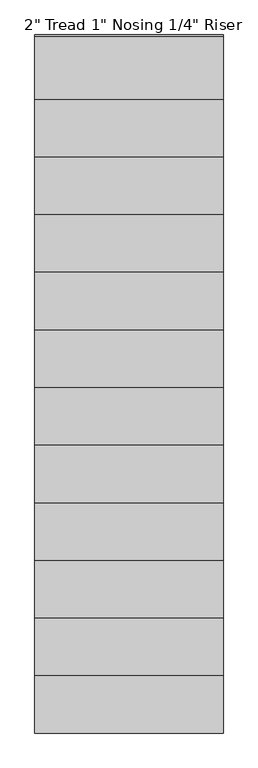
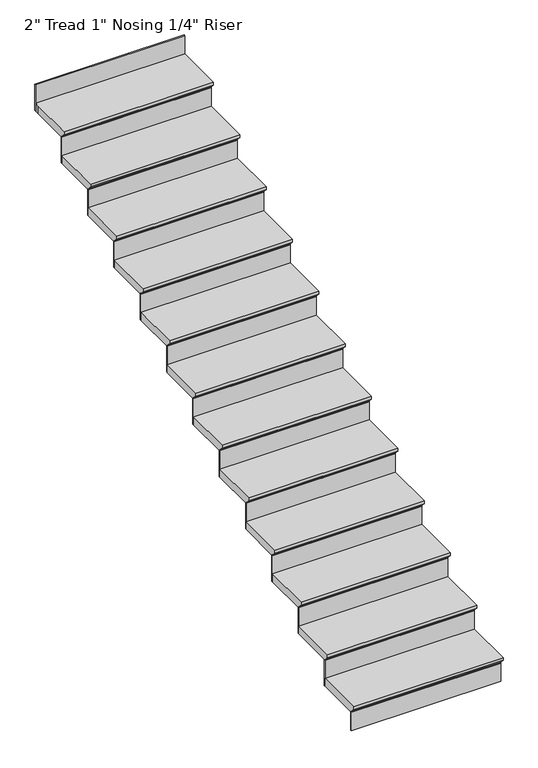
"""IFC4 building model written with IfcOpenShell, lengths in millimetres: stair flight geometry."""

from ifc_helpers import new_model, si_unit, origin, place, context, project, spatial, faceted_brep, source, transform, mapped, element, save


def stair_flight_de60d348(model_context):
    return source(origin(), model_context, "Body", "Brep", [
        faceted_brep([(-8119.8823175, 1898.2635177, 150.2833333), (-8119.8823175, 1898.2635177, 169.3333333), (-9034.2823175, 1898.2635177, 169.3333333), (-9034.2823175, 1898.2635177, 150.2833333), (-8119.8823175, 1923.6635177, 124.8833333), (-9034.2823175, 1923.6635177, 124.8833333), (-8119.8823175, 2203.0635177, 169.3333333), (-9034.2823175, 2203.0635177, 169.3333333), (-9034.2823175, 1923.6635177, 118.5333333), (-9034.2823175, 2203.0635177, 118.5333333), (-8119.8823175, 2203.0635177, 118.5333333), (-8119.8823175, 1923.6635177, 118.5333333)], [[[0, 1, 2, 3]], [[4, 0, 3, 5]], [[2, 1, 6, 7]], [[8, 9, 10, 11]], [[2, 7, 9, 8, 5, 3]], [[8, 11, 4, 5]], [[6, 1, 0, 4, 11, 10]], [[7, 6, 10, 9]]]),
        faceted_brep([(-8119.8823175, 1923.6635177, 118.5333333), (-8119.8823175, 1923.6635177, 0.0), (-8119.8823175, 1930.0135177, 0.0), (-8119.8823175, 1930.0135177, 118.5333333), (-9034.2823175, 1923.6635177, 118.5333333), (-9034.2823175, 1930.0135177, 118.5333333), (-9034.2823175, 1930.0135177, 0.0), (-9034.2823175, 1923.6635177, 0.0)], [[[0, 1, 2, 3]], [[4, 5, 6, 7]], [[1, 0, 4, 7]], [[2, 1, 7, 6]], [[3, 2, 6, 5]], [[0, 3, 5, 4]]]),
        faceted_brep([(-8119.8823175, 2203.0635177, 287.8666667), (-8119.8823175, 2203.0635177, 118.5333333), (-8119.8823175, 2209.4135177, 118.5333333), (-8119.8823175, 2209.4135177, 287.8666667), (-9034.2823175, 2203.0635177, 287.8666667), (-9034.2823175, 2209.4135177, 287.8666667), (-9034.2823175, 2209.4135177, 118.5333333), (-9034.2823175, 2203.0635177, 118.5333333)], [[[0, 1, 2, 3]], [[4, 5, 6, 7]], [[1, 0, 4, 7]], [[2, 1, 7, 6]], [[3, 2, 6, 5]], [[0, 3, 5, 4]]]),
        faceted_brep([(-9034.2823175, 2177.6635177, 338.6666667), (-8119.8823175, 2177.6635177, 338.6666667), (-8119.8823175, 2482.4635177, 338.6666667), (-9034.2823175, 2482.4635177, 338.6666667), (-9034.2823175, 2203.0635177, 287.8666667), (-9034.2823175, 2482.4635177, 287.8666667), (-8119.8823175, 2482.4635177, 287.8666667), (-8119.8823175, 2203.0635177, 287.8666667), (-9034.2823175, 2203.0635177, 294.2166667), (-9034.2823175, 2177.6635177, 319.6166667), (-8119.8823175, 2203.0635177, 294.2166667), (-8119.8823175, 2177.6635177, 319.6166667)], [[[0, 1, 2, 3]], [[4, 5, 6, 7]], [[0, 3, 5, 4, 8, 9]], [[4, 7, 10, 8]], [[2, 1, 11, 10, 7, 6]], [[3, 2, 6, 5]], [[11, 1, 0, 9]], [[10, 11, 9, 8]]]),
        faceted_brep([(-8119.8823175, 2482.4635177, 457.2), (-8119.8823175, 2482.4635177, 287.8666667), (-8119.8823175, 2488.8135177, 287.8666667), (-8119.8823175, 2488.8135177, 457.2), (-9034.2823175, 2482.4635177, 457.2), (-9034.2823175, 2488.8135177, 457.2), (-9034.2823175, 2488.8135177, 287.8666667), (-9034.2823175, 2482.4635177, 287.8666667)], [[[0, 1, 2, 3]], [[4, 5, 6, 7]], [[1, 0, 4, 7]], [[2, 1, 7, 6]], [[3, 2, 6, 5]], [[0, 3, 5, 4]]]),
        faceted_brep([(-9034.2823175, 2457.0635177, 508.0), (-8119.8823175, 2457.0635177, 508.0), (-8119.8823175, 2761.8635177, 508.0), (-9034.2823175, 2761.8635177, 508.0), (-9034.2823175, 2482.4635177, 457.2), (-9034.2823175, 2761.8635177, 457.2), (-8119.8823175, 2761.8635177, 457.2), (-8119.8823175, 2482.4635177, 457.2), (-9034.2823175, 2482.4635177, 463.55), (-9034.2823175, 2457.0635177, 488.95), (-8119.8823175, 2482.4635177, 463.55), (-8119.8823175, 2457.0635177, 488.95)], [[[0, 1, 2, 3]], [[4, 5, 6, 7]], [[0, 3, 5, 4, 8, 9]], [[4, 7, 10, 8]], [[2, 1, 11, 10, 7, 6]], [[3, 2, 6, 5]], [[11, 1, 0, 9]], [[10, 11, 9, 8]]]),
        faceted_brep([(-8119.8823175, 2761.8635177, 626.5333333), (-8119.8823175, 2761.8635177, 457.2), (-8119.8823175, 2768.2135177, 457.2), (-8119.8823175, 2768.2135177, 626.5333333), (-9034.2823175, 2761.8635177, 626.5333333), (-9034.2823175, 2768.2135177, 626.5333333), (-9034.2823175, 2768.2135177, 457.2), (-9034.2823175, 2761.8635177, 457.2)], [[[0, 1, 2, 3]], [[4, 5, 6, 7]], [[1, 0, 4, 7]], [[2, 1, 7, 6]], [[3, 2, 6, 5]], [[0, 3, 5, 4]]]),
        faceted_brep([(-9034.2823175, 2736.4635177, 677.3333333), (-8119.8823175, 2736.4635177, 677.3333333), (-8119.8823175, 3041.2635177, 677.3333333), (-9034.2823175, 3041.2635177, 677.3333333), (-9034.2823175, 2761.8635177, 626.5333333), (-9034.2823175, 3041.2635177, 626.5333333), (-8119.8823175, 3041.2635177, 626.5333333), (-8119.8823175, 2761.8635177, 626.5333333), (-9034.2823175, 2761.8635177, 632.8833333), (-9034.2823175, 2736.4635177, 658.2833333), (-8119.8823175, 2761.8635177, 632.8833333), (-8119.8823175, 2736.4635177, 658.2833333)], [[[0, 1, 2, 3]], [[4, 5, 6, 7]], [[0, 3, 5, 4, 8, 9]], [[4, 7, 10, 8]], [[2, 1, 11, 10, 7, 6]], [[3, 2, 6, 5]], [[11, 1, 0, 9]], [[10, 11, 9, 8]]]),
        faceted_brep([(-8119.8823175, 3041.2635177, 795.8666667), (-8119.8823175, 3041.2635177, 626.5333333), (-8119.8823175, 3047.6135177, 626.5333333), (-8119.8823175, 3047.6135177, 795.8666667), (-9034.2823175, 3041.2635177, 795.8666667), (-9034.2823175, 3047.6135177, 795.8666667), (-9034.2823175, 3047.6135177, 626.5333333), (-9034.2823175, 3041.2635177, 626.5333333)], [[[0, 1, 2, 3]], [[4, 5, 6, 7]], [[1, 0, 4, 7]], [[2, 1, 7, 6]], [[3, 2, 6, 5]], [[0, 3, 5, 4]]]),
        faceted_brep([(-9034.2823175, 3015.8635177, 846.6666667), (-8119.8823175, 3015.8635177, 846.6666667), (-8119.8823175, 3320.6635177, 846.6666667), (-9034.2823175, 3320.6635177, 846.6666667), (-9034.2823175, 3041.2635177, 795.8666667), (-9034.2823175, 3320.6635177, 795.8666667), (-8119.8823175, 3320.6635177, 795.8666667), (-8119.8823175, 3041.2635177, 795.8666667), (-9034.2823175, 3041.2635177, 802.2166667), (-9034.2823175, 3015.8635177, 827.6166667), (-8119.8823175, 3041.2635177, 802.2166667), (-8119.8823175, 3015.8635177, 827.6166667)], [[[0, 1, 2, 3]], [[4, 5, 6, 7]], [[0, 3, 5, 4, 8, 9]], [[4, 7, 10, 8]], [[2, 1, 11, 10, 7, 6]], [[3, 2, 6, 5]], [[11, 1, 0, 9]], [[10, 11, 9, 8]]]),
        faceted_brep([(-8119.8823175, 3320.6635177, 965.2), (-8119.8823175, 3320.6635177, 795.8666667), (-8119.8823175, 3327.0135177, 795.8666667), (-8119.8823175, 3327.0135177, 965.2), (-9034.2823175, 3320.6635177, 965.2), (-9034.2823175, 3327.0135177, 965.2), (-9034.2823175, 3327.0135177, 795.8666667), (-9034.2823175, 3320.6635177, 795.8666667)], [[[0, 1, 2, 3]], [[4, 5, 6, 7]], [[1, 0, 4, 7]], [[2, 1, 7, 6]], [[3, 2, 6, 5]], [[0, 3, 5, 4]]]),
        faceted_brep([(-9034.2823175, 3295.2635177, 1016.0), (-8119.8823175, 3295.2635177, 1016.0), (-8119.8823175, 3600.0635177, 1016.0), (-9034.2823175, 3600.0635177, 1016.0), (-9034.2823175, 3320.6635177, 965.2), (-9034.2823175, 3600.0635177, 965.2), (-8119.8823175, 3600.0635177, 965.2), (-8119.8823175, 3320.6635177, 965.2), (-9034.2823175, 3320.6635177, 971.55), (-9034.2823175, 3295.2635177, 996.95), (-8119.8823175, 3320.6635177, 971.55), (-8119.8823175, 3295.2635177, 996.95)], [[[0, 1, 2, 3]], [[4, 5, 6, 7]], [[0, 3, 5, 4, 8, 9]], [[4, 7, 10, 8]], [[2, 1, 11, 10, 7, 6]], [[3, 2, 6, 5]], [[11, 1, 0, 9]], [[10, 11, 9, 8]]]),
        faceted_brep([(-8119.8823175, 3600.0635177, 1134.5333333), (-8119.8823175, 3600.0635177, 965.2), (-8119.8823175, 3606.4135177, 965.2), (-8119.8823175, 3606.4135177, 1134.5333333), (-9034.2823175, 3600.0635177, 1134.5333333), (-9034.2823175, 3606.4135177, 1134.5333333), (-9034.2823175, 3606.4135177, 965.2), (-9034.2823175, 3600.0635177, 965.2)], [[[0, 1, 2, 3]], [[4, 5, 6, 7]], [[1, 0, 4, 7]], [[2, 1, 7, 6]], [[3, 2, 6, 5]], [[0, 3, 5, 4]]]),
        faceted_brep([(-9034.2823175, 3574.6635177, 1185.3333333), (-8119.8823175, 3574.6635177, 1185.3333333), (-8119.8823175, 3879.4635177, 1185.3333333), (-9034.2823175, 3879.4635177, 1185.3333333), (-9034.2823175, 3600.0635177, 1134.5333333), (-9034.2823175, 3879.4635177, 1134.5333333), (-8119.8823175, 3879.4635177, 1134.5333333), (-8119.8823175, 3600.0635177, 1134.5333333), (-9034.2823175, 3600.0635177, 1140.8833333), (-9034.2823175, 3574.6635177, 1166.2833333), (-8119.8823175, 3600.0635177, 1140.8833333), (-8119.8823175, 3574.6635177, 1166.2833333)], [[[0, 1, 2, 3]], [[4, 5, 6, 7]], [[0, 3, 5, 4, 8, 9]], [[4, 7, 10, 8]], [[2, 1, 11, 10, 7, 6]], [[3, 2, 6, 5]], [[11, 1, 0, 9]], [[10, 11, 9, 8]]]),
        faceted_brep([(-8119.8823175, 3879.4635177, 1303.8666667), (-8119.8823175, 3879.4635177, 1134.5333333), (-8119.8823175, 3885.8135177, 1134.5333333), (-8119.8823175, 3885.8135177, 1303.8666667), (-9034.2823175, 3879.4635177, 1303.8666667), (-9034.2823175, 3885.8135177, 1303.8666667), (-9034.2823175, 3885.8135177, 1134.5333333), (-9034.2823175, 3879.4635177, 1134.5333333)], [[[0, 1, 2, 3]], [[4, 5, 6, 7]], [[1, 0, 4, 7]], [[2, 1, 7, 6]], [[3, 2, 6, 5]], [[0, 3, 5, 4]]]),
        faceted_brep([(-9034.2823175, 3854.0635177, 1354.6666667), (-8119.8823175, 3854.0635177, 1354.6666667), (-8119.8823175, 4158.8635177, 1354.6666667), (-9034.2823175, 4158.8635177, 1354.6666667), (-9034.2823175, 3879.4635177, 1303.8666667), (-9034.2823175, 4158.8635177, 1303.8666667), (-8119.8823175, 4158.8635177, 1303.8666667), (-8119.8823175, 3879.4635177, 1303.8666667), (-9034.2823175, 3879.4635177, 1310.2166667), (-9034.2823175, 3854.0635177, 1335.6166667), (-8119.8823175, 3879.4635177, 1310.2166667), (-8119.8823175, 3854.0635177, 1335.6166667)], [[[0, 1, 2, 3]], [[4, 5, 6, 7]], [[0, 3, 5, 4, 8, 9]], [[4, 7, 10, 8]], [[2, 1, 11, 10, 7, 6]], [[3, 2, 6, 5]], [[11, 1, 0, 9]], [[10, 11, 9, 8]]]),
        faceted_brep([(-8119.8823175, 4158.8635177, 1473.2), (-8119.8823175, 4158.8635177, 1303.8666667), (-8119.8823175, 4165.2135177, 1303.8666667), (-8119.8823175, 4165.2135177, 1473.2), (-9034.2823175, 4158.8635177, 1473.2), (-9034.2823175, 4165.2135177, 1473.2), (-9034.2823175, 4165.2135177, 1303.8666667), (-9034.2823175, 4158.8635177, 1303.8666667)], [[[0, 1, 2, 3]], [[4, 5, 6, 7]], [[1, 0, 4, 7]], [[2, 1, 7, 6]], [[3, 2, 6, 5]], [[0, 3, 5, 4]]]),
        faceted_brep([(-9034.2823175, 4133.4635177, 1524.0), (-8119.8823175, 4133.4635177, 1524.0), (-8119.8823175, 4438.2635177, 1524.0), (-9034.2823175, 4438.2635177, 1524.0), (-9034.2823175, 4158.8635177, 1473.2), (-9034.2823175, 4438.2635177, 1473.2), (-8119.8823175, 4438.2635177, 1473.2), (-8119.8823175, 4158.8635177, 1473.2), (-9034.2823175, 4158.8635177, 1479.55), (-9034.2823175, 4133.4635177, 1504.95), (-8119.8823175, 4158.8635177, 1479.55), (-8119.8823175, 4133.4635177, 1504.95)], [[[0, 1, 2, 3]], [[4, 5, 6, 7]], [[0, 3, 5, 4, 8, 9]], [[4, 7, 10, 8]], [[2, 1, 11, 10, 7, 6]], [[3, 2, 6, 5]], [[11, 1, 0, 9]], [[10, 11, 9, 8]]]),
        faceted_brep([(-8119.8823175, 4438.2635177, 1642.5333333), (-8119.8823175, 4438.2635177, 1473.2), (-8119.8823175, 4444.6135177, 1473.2), (-8119.8823175, 4444.6135177, 1642.5333333), (-9034.2823175, 4438.2635177, 1642.5333333), (-9034.2823175, 4444.6135177, 1642.5333333), (-9034.2823175, 4444.6135177, 1473.2), (-9034.2823175, 4438.2635177, 1473.2)], [[[0, 1, 2, 3]], [[4, 5, 6, 7]], [[1, 0, 4, 7]], [[2, 1, 7, 6]], [[3, 2, 6, 5]], [[0, 3, 5, 4]]]),
        faceted_brep([(-9034.2823175, 4412.8635177, 1693.3333333), (-8119.8823175, 4412.8635177, 1693.3333333), (-8119.8823175, 4717.6635177, 1693.3333333), (-9034.2823175, 4717.6635177, 1693.3333333), (-9034.2823175, 4438.2635177, 1642.5333333), (-9034.2823175, 4717.6635177, 1642.5333333), (-8119.8823175, 4717.6635177, 1642.5333333), (-8119.8823175, 4438.2635177, 1642.5333333), (-9034.2823175, 4438.2635177, 1648.8833333), (-9034.2823175, 4412.8635177, 1674.2833333), (-8119.8823175, 4438.2635177, 1648.8833333), (-8119.8823175, 4412.8635177, 1674.2833333)], [[[0, 1, 2, 3]], [[4, 5, 6, 7]], [[0, 3, 5, 4, 8, 9]], [[4, 7, 10, 8]], [[2, 1, 11, 10, 7, 6]], [[3, 2, 6, 5]], [[11, 1, 0, 9]], [[10, 11, 9, 8]]]),
        faceted_brep([(-8119.8823175, 4717.6635177, 1811.8666667), (-8119.8823175, 4717.6635177, 1642.5333333), (-8119.8823175, 4724.0135177, 1642.5333333), (-8119.8823175, 4724.0135177, 1811.8666667), (-9034.2823175, 4717.6635177, 1811.8666667), (-9034.2823175, 4724.0135177, 1811.8666667), (-9034.2823175, 4724.0135177, 1642.5333333), (-9034.2823175, 4717.6635177, 1642.5333333)], [[[0, 1, 2, 3]], [[4, 5, 6, 7]], [[1, 0, 4, 7]], [[2, 1, 7, 6]], [[3, 2, 6, 5]], [[0, 3, 5, 4]]]),
        faceted_brep([(-9034.2823175, 4692.2635177, 1862.6666667), (-8119.8823175, 4692.2635177, 1862.6666667), (-8119.8823175, 4997.0635177, 1862.6666667), (-9034.2823175, 4997.0635177, 1862.6666667), (-9034.2823175, 4717.6635177, 1811.8666667), (-9034.2823175, 4997.0635177, 1811.8666667), (-8119.8823175, 4997.0635177, 1811.8666667), (-8119.8823175, 4717.6635177, 1811.8666667), (-9034.2823175, 4717.6635177, 1818.2166667), (-9034.2823175, 4692.2635177, 1843.6166667), (-8119.8823175, 4717.6635177, 1818.2166667), (-8119.8823175, 4692.2635177, 1843.6166667)], [[[0, 1, 2, 3]], [[4, 5, 6, 7]], [[0, 3, 5, 4, 8, 9]], [[4, 7, 10, 8]], [[2, 1, 11, 10, 7, 6]], [[3, 2, 6, 5]], [[11, 1, 0, 9]], [[10, 11, 9, 8]]]),
        faceted_brep([(-8119.8823175, 5276.4635177, 2150.5333333), (-8119.8823175, 5276.4635177, 1981.2), (-8119.8823175, 5282.8135177, 1981.2), (-8119.8823175, 5282.8135177, 2150.5333333), (-9034.2823175, 5276.4635177, 2150.5333333), (-9034.2823175, 5282.8135177, 2150.5333333), (-9034.2823175, 5282.8135177, 1981.2), (-9034.2823175, 5276.4635177, 1981.2)], [[[0, 1, 2, 3]], [[4, 5, 6, 7]], [[1, 0, 4, 7]], [[2, 1, 7, 6]], [[3, 2, 6, 5]], [[0, 3, 5, 4]]]),
        faceted_brep([(-8119.8823175, 4997.0635177, 1981.2), (-8119.8823175, 4997.0635177, 1811.8666667), (-8119.8823175, 5003.4135177, 1811.8666667), (-8119.8823175, 5003.4135177, 1981.2), (-9034.2823175, 4997.0635177, 1981.2), (-9034.2823175, 5003.4135177, 1981.2), (-9034.2823175, 5003.4135177, 1811.8666667), (-9034.2823175, 4997.0635177, 1811.8666667)], [[[0, 1, 2, 3]], [[4, 5, 6, 7]], [[1, 0, 4, 7]], [[2, 1, 7, 6]], [[3, 2, 6, 5]], [[0, 3, 5, 4]]]),
        faceted_brep([(-9034.2823175, 5276.4635177, 2032.0), (-9034.2823175, 5251.0635177, 2032.0), (-9034.2823175, 4971.6635177, 2032.0), (-8119.8823175, 4971.6635177, 2032.0), (-8119.8823175, 5251.0635177, 2032.0), (-8119.8823175, 5276.4635177, 2032.0), (-9034.2823175, 5251.0635177, 1981.2), (-9034.2823175, 5276.4635177, 1981.2), (-8119.8823175, 5276.4635177, 1981.2), (-8119.8823175, 5251.0635177, 1981.2), (-8119.8823175, 4997.0635177, 1981.2), (-9034.2823175, 4997.0635177, 1981.2), (-9034.2823175, 4997.0635177, 1987.55), (-9034.2823175, 4971.6635177, 2012.95), (-8119.8823175, 4997.0635177, 1987.55), (-8119.8823175, 4971.6635177, 2012.95)], [[[0, 1, 2, 3, 4, 5]], [[6, 7, 8, 9, 10, 11]], [[1, 0, 7, 6]], [[2, 1, 6, 11, 12, 13]], [[11, 10, 14, 12]], [[4, 3, 15, 14, 10, 9]], [[5, 4, 9, 8]], [[0, 5, 8, 7]], [[15, 3, 2, 13]], [[14, 15, 13, 12]]]),
    ])


if __name__ == "__main__":
    model = new_model("IFC4")
    model_context = context("Model", 3, world=origin())
    ifc_project = project(units=[si_unit("LENGTHUNIT", "METRE", prefix="MILLI")], contexts=[model_context])
    site = spatial("IfcSite", under=ifc_project)
    building = spatial("IfcBuilding", under=site)
    placement = place(None, origin())
    stair_flight_shape = stair_flight_de60d348(model_context)
    element("IfcStairFlight", 1, ObjectType="2\" Tread 1\" Nosing 1/4\" Riser", at=placement, inside=building, context=model_context, shape_type="MappedRepresentation", body=[
        mapped(stair_flight_shape, transform((0.0, 0.0, 0.0), x_axis=(1.0, 0.0, 0.0), y_axis=(0.0, 1.0, 0.0), z_axis=(0.0, 0.0, 1.0))),
    ])
    save(model, "model.ifc")
